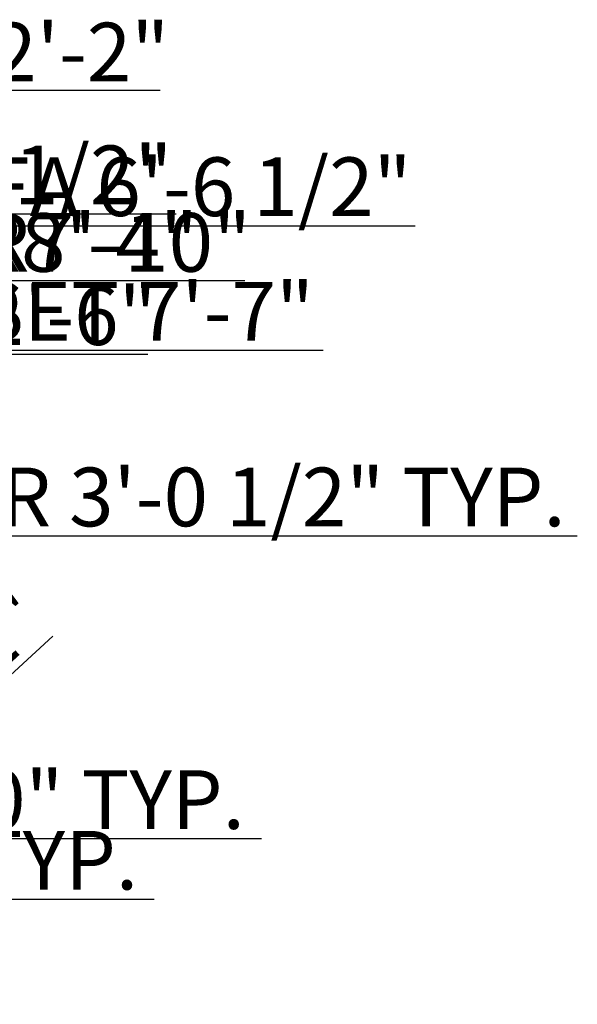
# Model space of a CAD drawing. Units: inches. Extents: x -299 to 1164, y -2 to 940.
# Tile 11 of 11: x 822 to 1164, y 108 to 712. Entities that reach past the tile are written whole.
import ezdxf

# ---------------------------------------------------------------- set-up
doc = ezdxf.new("R2010")
doc.units = ezdxf.units.IN
doc.layers.add('dimensions', color=191, linetype='Continuous', lineweight=18)
doc.styles.get("Standard").update_dxf_attribs({"font": 'arial.ttf'})
doc.dimstyles.new('ISO-25', dxfattribs={"dimtxt": 36, "dimasz": 36, "dimexe": 1.25, "dimexo": 0.625, "dimtad": 1, "dimlunit": 3, "dimtxsty": 'Standard', "dimcen": 2.5, "dimazin": 0, "dimtfac": 1, "dimtmove": 0, "dimatfit": 3, "dimfxl": 1, "dimarcsym": 0})

# ---------------------------------------------------------------- blocks, each defined once
blk = doc.blocks.new('*D19')
at = {"layer": 'Defpoints', "color": 0, "transparency": 16777216}
for p in [(449.18, 602.94), (514.78, 602.94), (514.78, 593.1)]:
    blk.add_point(p, dxfattribs=at)
at = {"layer": 'dimensions', "color": 0, "lineweight": -2, "transparency": 16777216}
for p, q in [((449.18, 602.31), (449.18, 591.85)), ((514.78, 602.31), (514.78, 591.85)), ((413.18, 593.1), (377.18, 593.1)), ((449.18, 593.1), (514.78, 593.1)), ((550.78, 593.1), (918.34, 593.1))]:
    blk.add_line(p, q, dxfattribs=at)
at = {"layer": 'dimensions', "color": 0, "transparency": 16777216}
for points in [[(413.18, 599.1), (413.18, 587.1), (449.18, 593.1)], [(550.78, 599.1), (550.78, 587.1), (514.78, 593.1)]]:
    blk.add_solid(points, dxfattribs=at)
at = {"layer": 'dimensions', "color": 0, "transparency": 16777216, "insert": (752.56, 612.35), "char_height": 36, "attachment_point": 5}
blk.add_mtext('SOFA 5\'-5 1/2"', dxfattribs=at)
blk = doc.blocks.new('*D21')
at = {"layer": 'Defpoints', "color": 0, "transparency": 16777216}
for p in [(618.72, 597.64), (697.42, 597.64), (697.42, 585.83)]:
    blk.add_point(p, dxfattribs=at)
at = {"layer": 'dimensions', "color": 0, "lineweight": -2, "transparency": 16777216}
for p, q in [((618.72, 597.01), (618.72, 584.58)), ((697.42, 597.01), (697.42, 584.58)), ((654.72, 585.83), (661.42, 585.83)), ((697.42, 585.83), (1064.98, 585.83))]:
    blk.add_line(p, q, dxfattribs=at)
at = {"layer": 'dimensions', "color": 0, "transparency": 16777216}
for points in [[(654.72, 591.83), (654.72, 579.83), (618.72, 585.83)], [(661.42, 591.83), (661.42, 579.83), (697.42, 585.83)]]:
    blk.add_solid(points, dxfattribs=at)
at = {"layer": 'dimensions', "color": 0, "transparency": 16777216, "insert": (899.2, 605.08), "char_height": 36, "attachment_point": 5}
blk.add_mtext('SOFA 6\'-6 1/2"', dxfattribs=at)
blk = doc.blocks.new('*D24')
at = {"layer": 'Defpoints', "color": 0, "transparency": 16777216}
for p in [(701.12, 517.34), (731.32, 517.34), (731.32, 506.96)]:
    blk.add_point(p, dxfattribs=at)
at = {"layer": 'dimensions', "color": 0, "lineweight": -2, "transparency": 16777216}
for p, q in [((701.12, 516.71), (701.12, 505.71)), ((731.32, 516.71), (731.32, 505.71)), ((665.12, 506.96), (629.12, 506.96)), ((701.12, 506.96), (731.32, 506.96)), ((767.32, 506.96), (900.88, 506.96))]:
    blk.add_line(p, q, dxfattribs=at)
at = {"layer": 'dimensions', "color": 0, "transparency": 16777216}
for points in [[(665.12, 512.96), (665.12, 500.96), (701.12, 506.96)], [(767.32, 512.96), (767.32, 500.96), (731.32, 506.96)]]:
    blk.add_solid(points, dxfattribs=at)
at = {"layer": 'dimensions', "color": 0, "transparency": 16777216, "insert": (852.1, 525.97), "char_height": 36, "attachment_point": 5}
blk.add_mtext('2\'-6"', dxfattribs=at)
blk = doc.blocks.new('*D29')
at = {"layer": 'Defpoints', "color": 0, "transparency": 16777216}
for p in [(304.07, 183.49), (376.07, 183.49), (376.07, 172.69)]:
    blk.add_point(p, dxfattribs=at)
at = {"layer": 'dimensions', "color": 0, "lineweight": -2, "transparency": 16777216}
for p, q in [((304.07, 182.86), (304.07, 171.44)), ((376.07, 182.86), (376.07, 171.44)), ((268.07, 172.69), (232.07, 172.69)), ((304.07, 172.69), (376.07, 172.69)), ((412.07, 172.69), (904.87, 172.69))]:
    blk.add_line(p, q, dxfattribs=at)
at = {"layer": 'dimensions', "color": 0, "transparency": 16777216}
for points in [[(268.07, 178.69), (268.07, 166.69), (304.07, 172.69)], [(412.07, 178.69), (412.07, 166.69), (376.07, 172.69)]]:
    blk.add_solid(points, dxfattribs=at)
at = {"layer": 'dimensions', "color": 0, "transparency": 16777216, "insert": (676.47, 191.94), "char_height": 36, "attachment_point": 5}
blk.add_mtext('WINDOW 6\'-0" TYP.', dxfattribs=at)
blk = doc.blocks.new('*D33')
at = {"layer": 'Defpoints', "color": 0, "transparency": 16777216}
for p in [(419.84, 213.49), (443.84, 213.49), (443.84, 209.89)]:
    blk.add_point(p, dxfattribs=at)
at = {"layer": 'dimensions', "color": 0, "lineweight": -2, "transparency": 16777216}
for p, q in [((419.84, 212.86), (419.84, 208.64)), ((443.84, 212.86), (443.84, 208.64)), ((383.84, 209.89), (347.84, 209.89)), ((419.84, 209.89), (443.84, 209.89)), ((479.84, 209.89), (970.68, 209.89))]:
    blk.add_line(p, q, dxfattribs=at)
at = {"layer": 'dimensions', "color": 0, "transparency": 16777216}
for points in [[(383.84, 215.89), (383.84, 203.89), (419.84, 209.89)], [(479.84, 215.89), (479.84, 203.89), (443.84, 209.89)]]:
    blk.add_solid(points, dxfattribs=at)
at = {"layer": 'dimensions', "color": 0, "transparency": 16777216, "insert": (743.26, 229.13), "char_height": 36, "attachment_point": 5}
blk.add_mtext('GLAZING 2\'-0" TYP.', dxfattribs=at)
blk = doc.blocks.new('*D37')
at = {"layer": 'Defpoints', "color": 0, "transparency": 16777216}
for p in [(588.07, 400.99), (624.7, 400.99), (624.7, 395.5)]:
    blk.add_point(p, dxfattribs=at)
at = {"layer": 'dimensions', "color": 0, "lineweight": -2, "transparency": 16777216}
for p, q in [((588.07, 400.36), (588.07, 394.25)), ((624.7, 400.36), (624.7, 394.25)), ((552.07, 395.5), (516.07, 395.5)), ((588.07, 395.5), (624.7, 395.5)), ((660.7, 395.5), (1164.33, 395.5))]:
    blk.add_line(p, q, dxfattribs=at)
at = {"layer": 'dimensions', "color": 0, "transparency": 16777216}
for points in [[(552.07, 401.5), (552.07, 389.5), (588.07, 395.5)], [(660.7, 401.5), (660.7, 389.5), (624.7, 395.5)]]:
    blk.add_solid(points, dxfattribs=at)
at = {"layer": 'dimensions', "color": 0, "transparency": 16777216, "insert": (930.51, 414.76), "char_height": 36, "attachment_point": 5}
blk.add_mtext('DOOR 3\'-0 1/2" TYP.', dxfattribs=at)
blk = doc.blocks.new('*D39')
at = {"layer": 'Defpoints', "color": 0, "transparency": 16777216}
for p in [(575.6, 509.45), (484.6, 495.8), (575.6, 495.8)]:
    blk.add_point(p, dxfattribs=at)
at = {"layer": 'dimensions', "color": 0, "lineweight": -2, "transparency": 16777216}
for p, q in [((484.6, 496.43), (484.6, 510.7)), ((520.6, 509.45), (539.6, 509.45)), ((575.6, 496.43), (575.6, 510.7)), ((575.6, 509.45), (1008.53, 509.45))]:
    blk.add_line(p, q, dxfattribs=at)
at = {"layer": 'dimensions', "color": 0, "transparency": 16777216}
for points in [[(520.6, 515.45), (520.6, 503.45), (484.6, 509.45)], [(539.6, 515.45), (539.6, 503.45), (575.6, 509.45)]]:
    blk.add_solid(points, dxfattribs=at)
at = {"layer": 'dimensions', "color": 0, "transparency": 16777216, "insert": (810.07, 528.69), "char_height": 36, "attachment_point": 5}
blk.add_mtext('DINING SET 7\'-7"', dxfattribs=at)
blk = doc.blocks.new('*D51')
at = {"layer": 'Defpoints', "color": 0, "transparency": 16777216}
for p in [(739.07, 668.99), (713.07, 405.49), (739.07, 396.49)]:
    blk.add_point(p, dxfattribs=at)
at = {"layer": 'dimensions', "color": 0, "lineweight": -2, "transparency": 16777216}
for p, q in [((677.07, 668.99), (641.07, 668.99)), ((713.07, 406.11), (713.07, 670.24)), ((713.07, 668.99), (739.07, 668.99)), ((739.07, 397.11), (739.07, 670.24)), ((775.07, 668.99), (908.63, 668.99))]:
    blk.add_line(p, q, dxfattribs=at)
at = {"layer": 'dimensions', "color": 0, "transparency": 16777216}
for points in [[(677.07, 674.99), (677.07, 662.99), (713.07, 668.99)], [(775.07, 674.99), (775.07, 662.99), (739.07, 668.99)]]:
    blk.add_solid(points, dxfattribs=at)
at = {"layer": 'dimensions', "color": 0, "transparency": 16777216, "insert": (859.85, 687.69), "char_height": 36, "attachment_point": 5}
blk.add_mtext('2\'-2"', dxfattribs=at)
blk = doc.blocks.new('*D60')
at = {"layer": 'Defpoints', "color": 0, "transparency": 16777216}
for p in [(672.12, 177.62), (655.34, 162.24)]:
    blk.add_point(p, dxfattribs=at)
at = {"layer": 'dimensions', "color": 0, "lineweight": -2, "transparency": 16777216}
for p, q in [((842.68, 333.96), (698.66, 201.95)), ((655.34, 162.24), (672.12, 177.62))]:
    blk.add_line(p, q, dxfattribs=at)
at = {"layer": 'dimensions', "color": 0, "transparency": 16777216}
blk.add_solid([(694.61, 206.37), (702.71, 197.52), (672.12, 177.62)], dxfattribs=at)
at = {"layer": 'dimensions', "color": 0, "transparency": 16777216, "insert": (771.3, 293.9), "char_height": 36, "attachment_point": 5, "rotation": 42.51051}
blk.add_mtext('R1\'-11"', dxfattribs=at)
blk = doc.blocks.new('*D65')
at = {"layer": 'Defpoints', "color": 0, "transparency": 16777216}
for p in [(624.36, 551.93), (724.18, 551.93)]:
    blk.add_point(p, dxfattribs=at)
at = {"layer": 'dimensions', "color": 0, "lineweight": -2, "transparency": 16777216}
for p, q in [((624.36, 551.93), (724.18, 551.93)), ((927.58, 551.93), (760.18, 551.93))]:
    blk.add_line(p, q, dxfattribs=at)
at = {"layer": 'dimensions', "color": 0, "transparency": 16777216}
blk.add_solid([(760.18, 557.93), (760.18, 545.93), (724.18, 551.93)], dxfattribs=at)
at = {"layer": 'dimensions', "color": 0, "transparency": 16777216, "insert": (861.88, 570.93), "char_height": 36, "attachment_point": 5, "rotation": 0.00009}
blk.add_mtext('R8\'-4"', dxfattribs=at)
blk = doc.blocks.new('*D66')
at = {"layer": 'Defpoints', "color": 0, "transparency": 16777216}
for p in [(635.03, 551.93), (729.12, 551.93)]:
    blk.add_point(p, dxfattribs=at)
at = {"layer": 'dimensions', "color": 0, "lineweight": -2, "transparency": 16777216}
for p, q in [((635.03, 551.93), (729.12, 551.93)), ((960.49, 551.93), (765.12, 551.93))]:
    blk.add_line(p, q, dxfattribs=at)
at = {"layer": 'dimensions', "color": 0, "transparency": 16777216}
blk.add_solid([(765.12, 557.93), (765.12, 545.93), (729.12, 551.93)], dxfattribs=at)
at = {"layer": 'dimensions', "color": 0, "transparency": 16777216, "insert": (880.81, 570.93), "char_height": 36, "attachment_point": 5, "rotation": 0.0001}
blk.add_mtext('R7\'-10"', dxfattribs=at)

msp = doc.modelspace()

# ---------------------------------------------------------------- dimensions: what is measured, and where the dimension line sits
at = {"layer": 'dimensions'}
for base, p1, p2, picture, middle in [((739.071, 668.989), (713.071, 405.489), (739.071, 396.489), '*D51', (859.852, 687.688)), ((731.317, 506.96), (701.119, 517.338), (731.317, 517.338), '*D24', (852.097, 525.966))]:
    dim = msp.add_linear_dim(base=base, p1=p1, p2=p2, dimstyle='ISO-25', override={"dimdec": 1, "dimlfac": 1, "dimrnd": 0, "dimzin": 1, "dimdsep": 46, "dimlunit": 4, "dimfrac": 2}, dxfattribs=at)
    dim.commit()
    dim.dimension.update_dxf_attribs({"geometry": picture, "text_midpoint": middle})
for base, p1, p2, text, picture, middle in [((514.778, 593.095), (449.176, 602.936), (514.778, 602.936), 'SOFA <>', '*D19', (752.559, 612.347)), ((697.417, 585.833), (618.725, 597.637), (697.417, 597.637), 'SOFA <>', '*D21', (899.198, 605.084)), ((575.6, 509.45), (484.6, 495.8), (575.6, 495.8), 'DINING SET <>', '*D39', (810.066, 528.689)), ((624.698, 395.495), (588.071, 400.989), (624.698, 400.989), 'DOOR <> TYP.', '*D37', (930.512, 414.759)), ((443.844, 209.889), (419.844, 213.489), (443.844, 213.489), 'GLAZING <> TYP.', '*D33', (743.261, 229.128)), ((376.071, 172.689), (304.071, 183.489), (376.071, 183.489), 'WINDOW <> TYP.', '*D29', (676.471, 191.94))]:
    dim = msp.add_linear_dim(base=base, p1=p1, p2=p2, text=text, dimstyle='ISO-25', override={"dimdec": 1, "dimlfac": 1, "dimrnd": 0, "dimzin": 1, "dimdsep": 46, "dimlunit": 4, "dimfrac": 2}, dxfattribs=at)
    dim.commit()
    dim.dimension.update_dxf_attribs({"geometry": picture, "text_midpoint": middle})
for center, mpoint, picture, middle in [((624.364, 551.928), (724.179, 551.928), '*D65', (861.879, 570.934)), ((635.027, 551.928), (729.12, 551.928), '*D66', (880.805, 570.934)), ((655.344, 162.239), (672.123, 177.62), '*D60', (771.303, 293.901))]:
    dim = msp.add_radius_dim(center=center, mpoint=mpoint, dimstyle='ISO-25', override={"dimdec": 1, "dimlfac": 1, "dimrnd": 0, "dimzin": 1, "dimdsep": 46, "dimlunit": 4, "dimfrac": 2}, dxfattribs=at)
    dim.commit()
    dim.dimension.update_dxf_attribs({"geometry": picture, "text_midpoint": middle})

doc.saveas('drawing.dxf')
